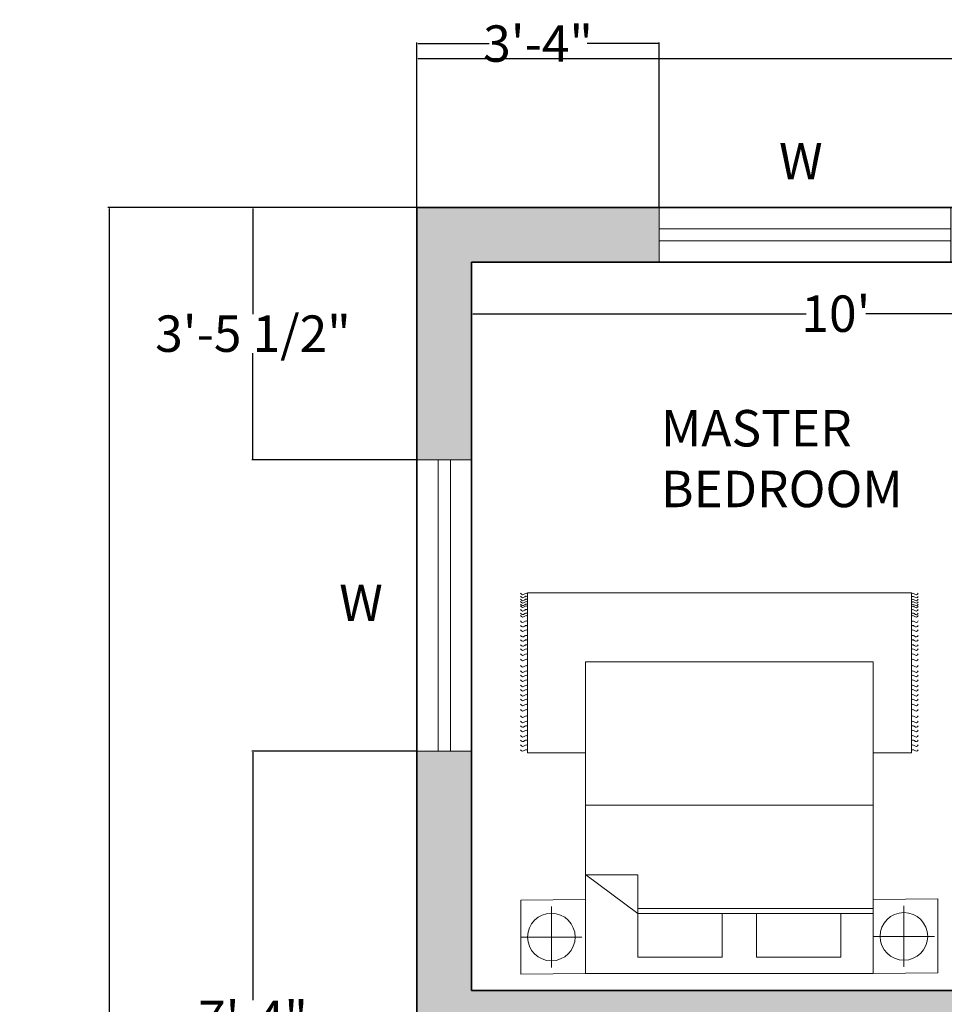
# Model space of a CAD drawing. Units: inches. Extents: x 302 to 1258, y 831 to 1373.
# Tile 3 of 13: x 302 to 455, y 1211 to 1373. Entities that reach past the tile are written whole.
import ezdxf

# ---------------------------------------------------------------- set-up
doc = ezdxf.new("R2010")
doc.units = ezdxf.units.IN
doc.header["$MEASUREMENT"] = 0
for name, color, linetype, lineweight in [('A-ANNO-DIMS', 2, 'Continuous', 18), ('A-ANNO-TEXT', 7, 'Continuous', 18), ('A-AREA-IDEN', 7, 'Continuous', 18), ('A-FURN', 8, 'Continuous', 18), ('A-GLAZ', 4, 'Continuous', 18), ('A-WALL', 7, 'Continuous', 35), ('A-WALL-PATT', 251, 'Continuous', 13)]:
    doc.layers.add(name, color=color, linetype=linetype, lineweight=lineweight)
doc.styles.get("Standard").update_dxf_attribs({"font": 'arial.ttf'})
doc.dimstyles.get("Standard").update_dxf_attribs({"dimtxt": 6, "dimasz": 0.18, "dimexe": 0.18, "dimexo": 0.0625, "dimgap": 0.09, "dimtad": 0, "dimtih": 1, "dimtoh": 1, "dimdec": 1, "dimzin": 0, "dimdsep": 46, "dimlunit": 3, "dimtxsty": 'Standard', "dimcen": 0.09, "dimadec": 0, "dimazin": 0, "dimtfac": 1, "dimtdec": 1, "dimtofl": 0, "dimtmove": 0, "dimatfit": 3, "dimfxl": 1, "dimtolj": 1, "dimtzin": 0, "dimarcsym": 0})

# ---------------------------------------------------------------- blocks, each defined once
blk = doc.blocks.new('*D3')
at = {"layer": 'A-ANNO-DIMS', "color": 0, "lineweight": -2, "transparency": 16777216}
for p, q in [((376.67, 1333.26), (376.67, 1324.65)), ((496.67, 1333.26), (496.67, 1324.65)), ((376.85, 1324.83), (431.77, 1324.83)), ((496.49, 1324.83), (441.57, 1324.83))]:
    blk.add_line(p, q, dxfattribs=at)
at = {"layer": 'A-ANNO-DIMS', "color": 0, "transparency": 16777216}
for points in [[(376.85, 1324.86), (376.85, 1324.8), (376.67, 1324.83)], [(496.49, 1324.86), (496.49, 1324.8), (496.67, 1324.83)]]:
    blk.add_solid(points, dxfattribs=at)
at = {"layer": 'Defpoints', "color": 0, "transparency": 16777216}
for p in [(376.67, 1333.32), (496.67, 1333.32), (496.67, 1324.83)]:
    blk.add_point(p, dxfattribs=at)
at = {"layer": 'A-ANNO-DIMS', "color": 0, "transparency": 16777216, "insert": (436.67, 1324.83), "char_height": 6, "attachment_point": 5}
blk.add_mtext("\\A1;10'", dxfattribs=at)
blk = doc.blocks.new('*D31')
at = {"layer": 'A-ANNO-DIMS', "color": 0, "lineweight": -2, "transparency": 16777216}
for p, q in [((367.67, 1342.38), (367.67, 1367.04)), ((367.85, 1366.86), (532.23, 1366.86)), ((724.49, 1366.86), (560.11, 1366.86)), ((724.67, 1342.38), (724.67, 1367.04))]:
    blk.add_line(p, q, dxfattribs=at)
at = {"layer": 'A-ANNO-DIMS', "color": 0, "transparency": 16777216}
for points in [[(367.85, 1366.89), (367.85, 1366.83), (367.67, 1366.86)], [(724.49, 1366.89), (724.49, 1366.83), (724.67, 1366.86)]]:
    blk.add_solid(points, dxfattribs=at)
at = {"layer": 'Defpoints', "color": 0, "transparency": 16777216}
for p in [(724.67, 1366.86), (367.67, 1342.32), (724.67, 1342.32)]:
    blk.add_point(p, dxfattribs=at)
at = {"layer": 'A-ANNO-DIMS', "color": 0, "transparency": 16777216, "insert": (546.17, 1366.86), "char_height": 6, "attachment_point": 5}
blk.add_mtext('\\A1;29\'-9.0"', dxfattribs=at)
blk = doc.blocks.new('*D32')
at = {"layer": 'A-ANNO-DIMS', "color": 0, "lineweight": -2, "transparency": 16777216}
for p, q in [((367.61, 1342.32), (316.79, 1342.32)), ((316.97, 1342.14), (316.97, 1107.72)), ((316.97, 867), (316.97, 1101.41)), ((367.61, 866.82), (316.79, 866.82))]:
    blk.add_line(p, q, dxfattribs=at)
at = {"layer": 'A-ANNO-DIMS', "color": 0, "transparency": 16777216}
for points in [[(316.94, 1342.14), (317, 1342.14), (316.97, 1342.32)], [(316.94, 867), (317, 867), (316.97, 866.82)]]:
    blk.add_solid(points, dxfattribs=at)
at = {"layer": 'Defpoints', "color": 0, "transparency": 16777216}
for p in [(367.67, 1342.32), (316.97, 866.82), (367.67, 866.82)]:
    blk.add_point(p, dxfattribs=at)
at = {"layer": 'A-ANNO-DIMS', "color": 0, "transparency": 16777216, "insert": (316.97, 1104.57), "char_height": 6, "attachment_point": 5}
blk.add_mtext('\\A1;39\'-7.5"', dxfattribs=at)
blk = doc.blocks.new('BED-DOUBLE-WITH-NIGHTSTANDS')
for p, q in [((1.12, 36.41), (1.12, 62.78)), ((1.12, 62.78), (64.36, 62.78)), ((64.36, 62.78), (64.36, 36.41)), ((10.66, 36.41), (1.12, 36.41)), ((64.36, 36.41), (58.06, 36.41)), ((10.66, 27.82), (58.08, 27.82)), ((19.27, 16.32), (10.71, 16.32)), ((19.32, 9.97), (10.71, 16.32)), ((19.27, 9.97), (19.27, 16.32)), ((5.06, 1.07), (5.06, 11.12)), ((19.27, 10.78), (58.08, 10.78)), ((19.32, 9.97), (58.08, 9.97)), ((63.11, 1.17), (63.11, 11.22)), ((0.03, 6.09), (10.09, 6.09)), ((58.08, 6.2), (68.14, 6.2))]:
    blk.add_line(p, q)
for points in [[(10.66, 0.1), (10.66, 51.42), (58.08, 51.42), (58.08, 0.1)], [(10.66, 12.29), (0.03, 12.19), (0.03, 0), (10.66, 0.1)], [(68.71, 12.39), (58.08, 12.29), (58.08, 0.1), (68.71, 0.2)], [(19.27, 2.8), (19.27, 9.97), (33.16, 9.97), (33.16, 2.8)], [(38.83, 2.8), (38.83, 9.97), (52.73, 9.97), (52.73, 2.8)]]:
    blk.add_lwpolyline(points, close=True)
for centre in [(5.06, 6.09), (63.11, 6.2)]:
    blk.add_circle(centre, 3.92)
for points, knots in [([(0, 62.71), (0.1, 62.59), (0.29, 62.35), (0.63, 62.59), (0.91, 62.76), (1.06, 62.66), (1.13, 62.61)], [0, 0, 0, 0, 0.400747, 0.791423, 1.067667, 1.29709, 1.29709, 1.29709, 1.29709]), ([(0, 62.24), (0.1, 62.12), (0.29, 61.88), (0.63, 62.12), (0.91, 62.29), (1.06, 62.18), (1.13, 62.13)], [0, 0, 0, 0, 0.400747, 0.791423, 1.067667, 1.29709, 1.29709, 1.29709, 1.29709]), ([(0, 61.75), (0.1, 61.63), (0.29, 61.39), (0.63, 61.63), (0.91, 61.8), (1.06, 61.7), (1.13, 61.65)], [0, 0, 0, 0, 0.400747, 0.791423, 1.067667, 1.29709, 1.29709, 1.29709, 1.29709]), ([(65.48, 62.71), (65.39, 62.59), (65.19, 62.35), (64.85, 62.59), (64.57, 62.76), (64.42, 62.66), (64.36, 62.61)], [0, 0, 0, 0, 0.400747, 0.791423, 1.067667, 1.29709, 1.29709, 1.29709, 1.29709]), ([(65.48, 62.21), (65.39, 62.09), (65.19, 61.85), (64.85, 62.09), (64.57, 62.26), (64.42, 62.15), (64.36, 62.11)], [0, 0, 0, 0, 0.400747, 0.791423, 1.067667, 1.29709, 1.29709, 1.29709, 1.29709]), ([(65.48, 61.72), (65.39, 61.6), (65.19, 61.36), (64.85, 61.6), (64.57, 61.78), (64.42, 61.67), (64.36, 61.62)], [0, 0, 0, 0, 0.400747, 0.791423, 1.067667, 1.29709, 1.29709, 1.29709, 1.29709]), ([(0, 61.35), (0.1, 61.23), (0.29, 60.99), (0.63, 61.23), (0.91, 61.41), (1.06, 61.3), (1.13, 61.25)], [0, 0, 0, 0, 0.400747, 0.791423, 1.067667, 1.29709, 1.29709, 1.29709, 1.29709]), ([(0, 60.94), (0.1, 60.81), (0.29, 60.58), (0.63, 60.81), (0.91, 60.99), (1.05, 60.89), (1.12, 60.84)], [0, 0, 0, 0, 0.400747, 0.791423, 1.067667, 1.283686, 1.283686, 1.283686, 1.283686]), ([(0, 60.63), (0.1, 60.51), (0.29, 60.27), (0.63, 60.51), (0.91, 60.68), (1.05, 60.58), (1.12, 60.53)], [0, 0, 0, 0, 0.400747, 0.791423, 1.067667, 1.283686, 1.283686, 1.283686, 1.283686]), ([(0, 60.05), (0.1, 59.93), (0.29, 59.69), (0.63, 59.93), (0.91, 60.1), (1.05, 60), (1.12, 59.96)], [0, 0, 0, 0, 0.400747, 0.791423, 1.067667, 1.283686, 1.283686, 1.283686, 1.283686]), ([(65.48, 61.33), (65.39, 61.21), (65.19, 60.97), (64.85, 61.21), (64.57, 61.38), (64.42, 61.27), (64.36, 61.22)], [0, 0, 0, 0, 0.400747, 0.791423, 1.067667, 1.29709, 1.29709, 1.29709, 1.29709]), ([(65.48, 60.91), (65.39, 60.79), (65.19, 60.55), (64.85, 60.79), (64.57, 60.96), (64.42, 60.85), (64.36, 60.81)], [0, 0, 0, 0, 0.400747, 0.791423, 1.067667, 1.29709, 1.29709, 1.29709, 1.29709]), ([(65.48, 60.6), (65.39, 60.48), (65.19, 60.24), (64.85, 60.48), (64.57, 60.65), (64.42, 60.54), (64.36, 60.5)], [0, 0, 0, 0, 0.400747, 0.791423, 1.067667, 1.29709, 1.29709, 1.29709, 1.29709]), ([(65.48, 60.03), (65.39, 59.9), (65.19, 59.67), (64.85, 59.9), (64.57, 60.08), (64.42, 59.97), (64.36, 59.92)], [0, 0, 0, 0, 0.400747, 0.791423, 1.067667, 1.29709, 1.29709, 1.29709, 1.29709]), ([(0, 59.46), (0.1, 59.34), (0.29, 59.09), (0.63, 59.34), (0.91, 59.51), (1.05, 59.41), (1.12, 59.36)], [0, 0, 0, 0, 0.402903, 0.794912, 1.071156, 1.287177, 1.287177, 1.287177, 1.287177]), ([(0, 59.03), (0.1, 58.91), (0.29, 58.67), (0.63, 58.91), (0.91, 59.08), (1.05, 58.98), (1.12, 58.93)], [0, 0, 0, 0, 0.400747, 0.791423, 1.067667, 1.283686, 1.283686, 1.283686, 1.283686]), ([(65.48, 59.46), (65.39, 59.33), (65.2, 59.08), (64.85, 59.34), (64.57, 59.51), (64.42, 59.4), (64.36, 59.36)], [0, 0, 0, 0, 0.407265, 0.802015, 1.07826, 1.307683, 1.307683, 1.307683, 1.307683]), ([(65.48, 59.03), (65.39, 58.91), (65.19, 58.67), (64.85, 58.91), (64.57, 59.08), (64.42, 58.97), (64.36, 58.93)], [0, 0, 0, 0, 0.400747, 0.791423, 1.067667, 1.29709, 1.29709, 1.29709, 1.29709]), ([(0, 58.15), (0.1, 58.03), (0.29, 57.79), (0.63, 58.03), (0.91, 58.2), (1.05, 58.1), (1.12, 58.05)], [0, 0, 0, 0, 0.400747, 0.791423, 1.067667, 1.283686, 1.283686, 1.283686, 1.283686]), ([(0, 57.42), (0.1, 57.3), (0.29, 57.06), (0.63, 57.3), (0.91, 57.47), (1.06, 57.36), (1.13, 57.32)], [0, 0, 0, 0, 0.400747, 0.791423, 1.067667, 1.29709, 1.29709, 1.29709, 1.29709]), ([(65.48, 58.15), (65.39, 58.03), (65.19, 57.79), (64.85, 58.03), (64.57, 58.2), (64.42, 58.09), (64.36, 58.04)], [0, 0, 0, 0, 0.400747, 0.791423, 1.067667, 1.29709, 1.29709, 1.29709, 1.29709]), ([(65.48, 57.42), (65.39, 57.3), (65.19, 57.06), (64.85, 57.3), (64.57, 57.47), (64.42, 57.36), (64.36, 57.32)], [0, 0, 0, 0, 0.400747, 0.791423, 1.067667, 1.29709, 1.29709, 1.29709, 1.29709]), ([(0, 56.67), (0.1, 56.55), (0.29, 56.31), (0.63, 56.55), (0.91, 56.72), (1.06, 56.61), (1.13, 56.56)], [0, 0, 0, 0, 0.400747, 0.791423, 1.067667, 1.29709, 1.29709, 1.29709, 1.29709]), ([(0, 55.78), (0.1, 55.66), (0.29, 55.42), (0.63, 55.66), (0.91, 55.84), (1.06, 55.73), (1.13, 55.68)], [0, 0, 0, 0, 0.400747, 0.791423, 1.067667, 1.29709, 1.29709, 1.29709, 1.29709]), ([(65.48, 56.67), (65.39, 56.55), (65.19, 56.31), (64.85, 56.55), (64.57, 56.72), (64.42, 56.61), (64.36, 56.56)], [0, 0, 0, 0, 0.400747, 0.791423, 1.067667, 1.29709, 1.29709, 1.29709, 1.29709]), ([(65.48, 55.78), (65.39, 55.66), (65.19, 55.42), (64.85, 55.66), (64.57, 55.84), (64.42, 55.73), (64.36, 55.68)], [0, 0, 0, 0, 0.400747, 0.791423, 1.067667, 1.29709, 1.29709, 1.29709, 1.29709]), ([(0, 55.06), (0.1, 54.94), (0.29, 54.7), (0.63, 54.94), (0.91, 55.11), (1.06, 55), (1.13, 54.95)], [0, 0, 0, 0, 0.400747, 0.791423, 1.067667, 1.29709, 1.29709, 1.29709, 1.29709]), ([(0, 54.24), (0.1, 54.12), (0.29, 53.88), (0.63, 54.12), (0.91, 54.29), (1.06, 54.19), (1.13, 54.14)], [0, 0, 0, 0, 0.400747, 0.791423, 1.067667, 1.29709, 1.29709, 1.29709, 1.29709]), ([(0, 53.55), (0.1, 53.43), (0.29, 53.19), (0.63, 53.43), (0.91, 53.6), (1.06, 53.5), (1.13, 53.45)], [0, 0, 0, 0, 0.400747, 0.791423, 1.067667, 1.29709, 1.29709, 1.29709, 1.29709]), ([(65.48, 55.06), (65.39, 54.94), (65.19, 54.7), (64.85, 54.94), (64.57, 55.11), (64.42, 55), (64.36, 54.95)], [0, 0, 0, 0, 0.400747, 0.791423, 1.067667, 1.29709, 1.29709, 1.29709, 1.29709]), ([(65.48, 54.24), (65.39, 54.12), (65.19, 53.88), (64.85, 54.12), (64.57, 54.29), (64.42, 54.19), (64.36, 54.14)], [0, 0, 0, 0, 0.400747, 0.791423, 1.067667, 1.29709, 1.29709, 1.29709, 1.29709]), ([(65.48, 53.55), (65.39, 53.43), (65.19, 53.19), (64.85, 53.43), (64.57, 53.6), (64.42, 53.5), (64.36, 53.45)], [0, 0, 0, 0, 0.400747, 0.791423, 1.067667, 1.29709, 1.29709, 1.29709, 1.29709]), ([(0, 52.73), (0.1, 52.61), (0.29, 52.37), (0.63, 52.61), (0.91, 52.79), (1.06, 52.68), (1.13, 52.63)], [0, 0, 0, 0, 0.400747, 0.791423, 1.067667, 1.29709, 1.29709, 1.29709, 1.29709]), ([(65.48, 52.73), (65.39, 52.61), (65.19, 52.37), (64.85, 52.61), (64.57, 52.79), (64.42, 52.68), (64.36, 52.63)], [0, 0, 0, 0, 0.400747, 0.791423, 1.067667, 1.29709, 1.29709, 1.29709, 1.29709]), ([(0, 51.85), (0.1, 51.73), (0.29, 51.49), (0.63, 51.73), (0.91, 51.9), (1.06, 51.8), (1.13, 51.75)], [0, 0, 0, 0, 0.400747, 0.791423, 1.067667, 1.29709, 1.29709, 1.29709, 1.29709]), ([(0, 50.82), (0.1, 50.69), (0.29, 50.46), (0.63, 50.69), (0.91, 50.87), (1.06, 50.76), (1.13, 50.71)], [0, 0, 0, 0, 0.400747, 0.791423, 1.067667, 1.29709, 1.29709, 1.29709, 1.29709]), ([(65.48, 51.85), (65.39, 51.73), (65.19, 51.49), (64.85, 51.73), (64.57, 51.9), (64.42, 51.8), (64.36, 51.75)], [0, 0, 0, 0, 0.400747, 0.791423, 1.067667, 1.29709, 1.29709, 1.29709, 1.29709]), ([(65.48, 50.82), (65.39, 50.69), (65.19, 50.46), (64.85, 50.69), (64.57, 50.87), (64.42, 50.76), (64.36, 50.71)], [0, 0, 0, 0, 0.400747, 0.791423, 1.067667, 1.29709, 1.29709, 1.29709, 1.29709]), ([(0, 49.93), (0.1, 49.81), (0.29, 49.57), (0.63, 49.81), (0.91, 49.99), (1.06, 49.88), (1.13, 49.83)], [0, 0, 0, 0, 0.400747, 0.791423, 1.067667, 1.29709, 1.29709, 1.29709, 1.29709]), ([(0, 49.21), (0.1, 49.08), (0.29, 48.84), (0.63, 49.08), (0.91, 49.26), (1.06, 49.15), (1.13, 49.1)], [0, 0, 0, 0, 0.400747, 0.791423, 1.067667, 1.29709, 1.29709, 1.29709, 1.29709]), ([(65.48, 49.93), (65.39, 49.81), (65.19, 49.57), (64.85, 49.81), (64.57, 49.99), (64.42, 49.88), (64.36, 49.83)], [0, 0, 0, 0, 0.400747, 0.791423, 1.067667, 1.29709, 1.29709, 1.29709, 1.29709]), ([(65.48, 49.21), (65.39, 49.08), (65.19, 48.84), (64.85, 49.08), (64.57, 49.26), (64.42, 49.15), (64.36, 49.1)], [0, 0, 0, 0, 0.400747, 0.791423, 1.067667, 1.29709, 1.29709, 1.29709, 1.29709]), ([(0, 48.45), (0.1, 48.33), (0.29, 48.09), (0.63, 48.33), (0.91, 48.51), (1.06, 48.4), (1.13, 48.35)], [0, 0, 0, 0, 0.400747, 0.791423, 1.067667, 1.29709, 1.29709, 1.29709, 1.29709]), ([(0, 47.57), (0.1, 47.45), (0.29, 47.21), (0.63, 47.45), (0.91, 47.62), (1.06, 47.52), (1.13, 47.47)], [0, 0, 0, 0, 0.400747, 0.791423, 1.067667, 1.29709, 1.29709, 1.29709, 1.29709]), ([(65.48, 48.45), (65.39, 48.33), (65.19, 48.09), (64.85, 48.33), (64.57, 48.51), (64.42, 48.4), (64.36, 48.35)], [0, 0, 0, 0, 0.400747, 0.791423, 1.067667, 1.29709, 1.29709, 1.29709, 1.29709]), ([(65.48, 47.57), (65.39, 47.45), (65.19, 47.21), (64.85, 47.45), (64.57, 47.62), (64.42, 47.52), (64.36, 47.47)], [0, 0, 0, 0, 0.400747, 0.791423, 1.067667, 1.29709, 1.29709, 1.29709, 1.29709]), ([(0, 46.84), (0.1, 46.72), (0.29, 46.48), (0.63, 46.72), (0.91, 46.89), (1.06, 46.79), (1.13, 46.74)], [0, 0, 0, 0, 0.400747, 0.791423, 1.067667, 1.29709, 1.29709, 1.29709, 1.29709]), ([(0, 46.03), (0.1, 45.91), (0.29, 45.67), (0.63, 45.91), (0.91, 46.08), (1.06, 45.97), (1.13, 45.92)], [0, 0, 0, 0, 0.400747, 0.791423, 1.067667, 1.29709, 1.29709, 1.29709, 1.29709]), ([(65.48, 46.84), (65.39, 46.72), (65.19, 46.48), (64.85, 46.72), (64.57, 46.89), (64.42, 46.79), (64.36, 46.74)], [0, 0, 0, 0, 0.400747, 0.791423, 1.067667, 1.29709, 1.29709, 1.29709, 1.29709]), ([(65.48, 46.03), (65.39, 45.91), (65.19, 45.67), (64.85, 45.91), (64.57, 46.08), (64.42, 45.97), (64.36, 45.92)], [0, 0, 0, 0, 0.400747, 0.791423, 1.067667, 1.29709, 1.29709, 1.29709, 1.29709]), ([(0, 45.25), (0.1, 45.13), (0.29, 44.89), (0.63, 45.13), (0.91, 45.3), (1.06, 45.2), (1.13, 45.15)], [0, 0, 0, 0, 0.400747, 0.791423, 1.067667, 1.29709, 1.29709, 1.29709, 1.29709]), ([(0, 44.43), (0.1, 44.31), (0.29, 44.07), (0.63, 44.31), (0.91, 44.49), (1.06, 44.38), (1.13, 44.33)], [0, 0, 0, 0, 0.400747, 0.791423, 1.067667, 1.29709, 1.29709, 1.29709, 1.29709]), ([(65.48, 45.25), (65.39, 45.13), (65.19, 44.89), (64.85, 45.13), (64.57, 45.3), (64.42, 45.2), (64.36, 45.15)], [0, 0, 0, 0, 0.400747, 0.791423, 1.067667, 1.29709, 1.29709, 1.29709, 1.29709]), ([(65.48, 44.43), (65.39, 44.31), (65.19, 44.07), (64.85, 44.31), (64.57, 44.49), (64.42, 44.38), (64.36, 44.33)], [0, 0, 0, 0, 0.400747, 0.791423, 1.067667, 1.29709, 1.29709, 1.29709, 1.29709]), ([(0, 43.55), (0.1, 43.43), (0.29, 43.19), (0.63, 43.43), (0.91, 43.6), (1.06, 43.5), (1.13, 43.45)], [0, 0, 0, 0, 0.400747, 0.791423, 1.067667, 1.29709, 1.29709, 1.29709, 1.29709]), ([(0, 42.52), (0.1, 42.39), (0.29, 42.15), (0.63, 42.39), (0.91, 42.57), (1.06, 42.46), (1.13, 42.41)], [0, 0, 0, 0, 0.400747, 0.791423, 1.067667, 1.29709, 1.29709, 1.29709, 1.29709]), ([(65.48, 43.55), (65.39, 43.43), (65.19, 43.19), (64.85, 43.43), (64.57, 43.6), (64.42, 43.5), (64.36, 43.45)], [0, 0, 0, 0, 0.400747, 0.791423, 1.067667, 1.29709, 1.29709, 1.29709, 1.29709]), ([(65.48, 42.52), (65.39, 42.39), (65.19, 42.15), (64.85, 42.39), (64.57, 42.57), (64.42, 42.46), (64.36, 42.41)], [0, 0, 0, 0, 0.400747, 0.791423, 1.067667, 1.29709, 1.29709, 1.29709, 1.29709]), ([(0, 41.63), (0.1, 41.51), (0.29, 41.27), (0.63, 41.51), (0.91, 41.68), (1.06, 41.58), (1.13, 41.53)], [0, 0, 0, 0, 0.400747, 0.791423, 1.067667, 1.29709, 1.29709, 1.29709, 1.29709]), ([(0, 40.9), (0.1, 40.78), (0.29, 40.54), (0.63, 40.78), (0.91, 40.96), (1.06, 40.85), (1.13, 40.8)], [0, 0, 0, 0, 0.400747, 0.791423, 1.067667, 1.29709, 1.29709, 1.29709, 1.29709]), ([(65.48, 41.63), (65.39, 41.51), (65.19, 41.27), (64.85, 41.51), (64.57, 41.68), (64.42, 41.58), (64.36, 41.53)], [0, 0, 0, 0, 0.400747, 0.791423, 1.067667, 1.29709, 1.29709, 1.29709, 1.29709]), ([(65.48, 40.9), (65.39, 40.78), (65.19, 40.54), (64.85, 40.78), (64.57, 40.96), (64.42, 40.85), (64.36, 40.8)], [0, 0, 0, 0, 0.400747, 0.791423, 1.067667, 1.29709, 1.29709, 1.29709, 1.29709]), ([(0, 40.15), (0.1, 40.03), (0.29, 39.79), (0.63, 40.03), (0.91, 40.2), (1.06, 40.1), (1.13, 40.05)], [0, 0, 0, 0, 0.400747, 0.791423, 1.067667, 1.29709, 1.29709, 1.29709, 1.29709]), ([(0, 39.27), (0.1, 39.15), (0.29, 38.91), (0.63, 39.15), (0.91, 39.32), (1.06, 39.22), (1.13, 39.17)], [0, 0, 0, 0, 0.400747, 0.791423, 1.067667, 1.29709, 1.29709, 1.29709, 1.29709]), ([(65.48, 40.15), (65.39, 40.03), (65.19, 39.79), (64.85, 40.03), (64.57, 40.2), (64.42, 40.1), (64.36, 40.05)], [0, 0, 0, 0, 0.400747, 0.791423, 1.067667, 1.29709, 1.29709, 1.29709, 1.29709]), ([(65.48, 39.27), (65.39, 39.15), (65.19, 38.91), (64.85, 39.15), (64.57, 39.32), (64.42, 39.22), (64.36, 39.17)], [0, 0, 0, 0, 0.400747, 0.791423, 1.067667, 1.29709, 1.29709, 1.29709, 1.29709]), ([(0, 38.54), (0.1, 38.42), (0.29, 38.18), (0.63, 38.42), (0.91, 38.59), (1.06, 38.49), (1.13, 38.44)], [0, 0, 0, 0, 0.400747, 0.791423, 1.067667, 1.29709, 1.29709, 1.29709, 1.29709]), ([(0, 37.73), (0.1, 37.61), (0.29, 37.37), (0.63, 37.61), (0.91, 37.78), (1.06, 37.67), (1.13, 37.62)], [0, 0, 0, 0, 0.400747, 0.791423, 1.067667, 1.29709, 1.29709, 1.29709, 1.29709]), ([(65.48, 38.54), (65.39, 38.42), (65.19, 38.18), (64.85, 38.42), (64.57, 38.59), (64.42, 38.49), (64.36, 38.44)], [0, 0, 0, 0, 0.400747, 0.791423, 1.067667, 1.29709, 1.29709, 1.29709, 1.29709]), ([(65.48, 37.73), (65.39, 37.61), (65.19, 37.37), (64.85, 37.61), (64.57, 37.78), (64.42, 37.67), (64.36, 37.62)], [0, 0, 0, 0, 0.400747, 0.791423, 1.067667, 1.29709, 1.29709, 1.29709, 1.29709]), ([(0, 36.95), (0.1, 36.83), (0.29, 36.59), (0.63, 36.83), (0.91, 37), (1.06, 36.89), (1.13, 36.85)], [0, 0, 0, 0, 0.400747, 0.791423, 1.067667, 1.29709, 1.29709, 1.29709, 1.29709]), ([(65.48, 36.95), (65.39, 36.83), (65.19, 36.59), (64.85, 36.83), (64.57, 37), (64.42, 36.89), (64.36, 36.85)], [0, 0, 0, 0, 0.400747, 0.791423, 1.067667, 1.29709, 1.29709, 1.29709, 1.29709])]:
    blk.add_open_spline(points, degree=3, knots=knots)
blk = doc.blocks.new('WINDOW-48IN')
for p, q in [((0, 0), (0, 9)), ((0, 9), (48, 9)), ((48, 9), (48, 0)), ((0, 5.5), (48, 5.5)), ((48, 3.5), (0, 3.5)), ((48, 0), (0, 0))]:
    blk.add_line(p, q)
blk = doc.blocks.new('*D69')
at = {"layer": 'A-ANNO-DIMS', "color": 0, "lineweight": -2, "transparency": 16777216}
for p, q in [((367.67, 1342.38), (367.67, 1369.5)), ((367.85, 1369.32), (379.56, 1369.32)), ((407.39, 1369.32), (395.68, 1369.32)), ((407.57, 1342.38), (407.57, 1369.5))]:
    blk.add_line(p, q, dxfattribs=at)
at = {"layer": 'A-ANNO-DIMS', "color": 0, "transparency": 16777216}
for points in [[(367.85, 1369.35), (367.85, 1369.29), (367.67, 1369.32)], [(407.39, 1369.35), (407.39, 1369.29), (407.57, 1369.32)]]:
    blk.add_solid(points, dxfattribs=at)
at = {"layer": 'Defpoints', "color": 0, "transparency": 16777216}
for p in [(407.57, 1369.32), (367.67, 1342.32), (407.57, 1342.32)]:
    blk.add_point(p, dxfattribs=at)
at = {"layer": 'A-ANNO-DIMS', "color": 0, "transparency": 16777216, "insert": (387.62, 1369.32), "char_height": 6, "attachment_point": 5}
blk.add_mtext('\\A1;3\'-4"', dxfattribs=at)
blk = doc.blocks.new('*D71')
at = {"layer": 'A-ANNO-DIMS', "color": 0, "lineweight": -2, "transparency": 16777216}
for p, q in [((367.61, 1342.32), (340.49, 1342.32)), ((340.67, 1342.14), (340.67, 1324.73)), ((340.67, 1300.94), (340.67, 1318.34)), ((367.61, 1300.76), (340.49, 1300.76))]:
    blk.add_line(p, q, dxfattribs=at)
at = {"layer": 'A-ANNO-DIMS', "color": 0, "transparency": 16777216}
for points in [[(340.64, 1342.14), (340.7, 1342.14), (340.67, 1342.32)], [(340.64, 1300.94), (340.7, 1300.94), (340.67, 1300.76)]]:
    blk.add_solid(points, dxfattribs=at)
at = {"layer": 'Defpoints', "color": 0, "transparency": 16777216}
for p in [(367.67, 1342.32), (340.67, 1300.76), (367.67, 1300.76)]:
    blk.add_point(p, dxfattribs=at)
at = {"layer": 'A-ANNO-DIMS', "color": 0, "transparency": 16777216, "insert": (340.67, 1321.54), "char_height": 6, "attachment_point": 5}
blk.add_mtext('\\A1;3\'-5 1/2"', dxfattribs=at)
blk = doc.blocks.new('*D72')
at = {"layer": 'A-ANNO-DIMS', "color": 0, "lineweight": -2, "transparency": 16777216}
for p, q in [((367.60766, 1252.758966), (340.49016, 1252.758966)), ((340.67016, 1252.578966), (340.67016, 1211.744211)), ((340.67016, 1164.729456), (340.67016, 1205.564211)), ((367.60766, 1164.549456), (340.49016, 1164.549456))]:
    blk.add_line(p, q, dxfattribs=at)
at = {"layer": 'A-ANNO-DIMS', "color": 0, "transparency": 16777216}
for points in [[(340.64016, 1252.578966), (340.70016, 1252.578966), (340.67016, 1252.758966)], [(340.64016, 1164.729456), (340.70016, 1164.729456), (340.67016, 1164.549456)]]:
    blk.add_solid(points, dxfattribs=at)
at = {"layer": 'Defpoints', "color": 0, "transparency": 16777216}
for p in [(367.67016, 1252.758966), (340.67016, 1164.549456), (367.67016, 1164.549456)]:
    blk.add_point(p, dxfattribs=at)
at = {"layer": 'A-ANNO-DIMS', "color": 0, "transparency": 16777216, "insert": (340.67016, 1208.654211), "char_height": 6, "attachment_point": 5}
blk.add_mtext('\\A1;7\'-4"', dxfattribs=at)

msp = doc.modelspace()

# ---------------------------------------------------------------- hatches: boundary and pattern name
at = {"layer": 'A-WALL-PATT'}
h = msp.add_hatch(color=256, dxfattribs=at)
h.dxf.hatch_style = 1
h.paths.add_polyline_path([(524.78, 1342.32), (455.57, 1342.32), (455.57, 1333.32), (496.67, 1333.32), (496.67, 1330.32), (501.17, 1330.32), (501.17, 1333.32), (524.78, 1333.32)])
h.paths.add_polyline_path([(724.67, 1342.32), (548.78, 1342.32), (548.78, 1333.32), (567.17, 1333.32), (567.17, 1213.32), (501.17, 1213.32), (501.17, 1306.32), (496.67, 1306.32), (496.67, 1213.32), (495.67, 1213.32), (495.67, 1208.82), (496.67, 1208.82), (572.67, 1208.82), (572.67, 1213.32), (571.67, 1213.32), (571.67, 1333.32), (715.67, 1333.32), (715.67, 1302.71), (724.67, 1302.71)])
h.paths.add_polyline_path([(376.67, 1333.32), (407.57, 1333.32), (407.57, 1342.32), (367.67, 1342.32), (367.67, 1300.76), (376.67, 1300.76)])
h.paths.add_polyline_path([(459.67, 1213.32), (376.67, 1213.32), (376.67, 1252.76), (367.67, 1252.76), (367.67, 1164.55), (376.67, 1164.55), (376.67, 1208.82), (454.67, 1208.82), (454.67, 1082.82), (459.17, 1082.82), (459.17, 1208.82), (459.67, 1208.82)])
h.paths.add_polyline_path([(376.67, 1116.55), (367.67, 1116.55), (367.67, 1024.44), (376.67, 1024.44)])
h.paths.add_polyline_path([(724.67, 1254.71), (715.67, 1254.71), (715.67, 1213.32), (608.67, 1213.32), (608.67, 1208.82), (615.17, 1208.82), (615.17, 1205.82), (619.67, 1205.82), (619.67, 1208.82), (715.67, 1208.82), (715.67, 1191.3), (724.67, 1191.3)])
h.paths.add_polyline_path([(724.67, 1167.3), (715.67, 1167.3), (715.67, 1136.82), (619.67, 1136.82), (619.67, 1181.82), (615.17, 1181.82), (615.17, 1136.82), (591.17, 1136.82), (591.17, 1129.32), (595.67, 1129.32), (595.67, 1132.32), (715.67, 1132.32), (715.67, 1097.42), (724.67, 1097.42)])
h.paths.add_polyline_path([(724.67, 1049.42), (715.67, 1049.42), (715.67, 1012.32), (595.67, 1012.32), (595.67, 1093.32), (591.17, 1093.32), (591.17, 1007.82), (715.67, 1007.82), (715.67, 875.82), (709.67, 875.82), (709.67, 866.82), (715.67, 866.82), (724.67, 866.82)])
h.paths.add_polyline_path([(673.67, 875.82), (623.88, 875.82), (623.88, 866.82), (673.67, 866.82)], flags=17)
h.paths.add_polyline_path([(575.88, 875.82), (477.17, 875.82), (477.17, 971.82), (472.67, 971.82), (472.67, 875.82), (376.67, 875.82), (376.67, 896.2), (367.67, 896.2), (367.67, 866.82), (575.88, 866.82)])
h.paths.add_polyline_path([(376.67, 976.44), (367.67, 976.44), (367.67, 944.2), (376.67, 944.2)])

# ---------------------------------------------------------------- linework, layer by layer
at = {"layer": 'A-WALL'}
for p, q in [((367.67, 1342.32), (724.67, 1342.32)), ((367.67, 1342.32), (367.67, 866.82)), ((376.67, 1333.32), (376.67, 1213.32)), ((376.67, 1333.32), (496.67, 1333.32)), ((376.67, 1213.32), (459.67, 1213.32))]:
    msp.add_line(p, q, dxfattribs=at)

# ---------------------------------------------------------------- block references
at = {"layer": 'A-FURN'}
msp.add_blockref('BED-DOUBLE-WITH-NIGHTSTANDS', (384.75, 1216.06), dxfattribs=at)
at = {"layer": 'A-GLAZ'}
msp.add_blockref('WINDOW-48IN', (407.57, 1333.32), dxfattribs=at)
at = {"layer": 'A-GLAZ', "rotation": 269.9999999999997}
msp.add_blockref('WINDOW-48IN', (367.67, 1300.76), dxfattribs=at)

# ---------------------------------------------------------------- texts
at = {"layer": 'A-ANNO-TEXT', "char_height": 6, "attachment_point": 1}
for insert in [(427.3, 1352.94), (354.87, 1280.2)]:
    msp.add_mtext_dynamic_manual_height_columns('W', width=16.4894, gutter_width=30, heights=[0], dxfattribs=dict(at, insert=insert))
at = {"layer": 'A-AREA-IDEN', "insert": (407.85, 1308.96), "char_height": 6, "attachment_point": 1}
msp.add_mtext_dynamic_manual_height_columns('MASTER\\PBEDROOM', width=60.4741, gutter_width=30, heights=[0], dxfattribs=at)

# ---------------------------------------------------------------- dimensions: what is measured, and where the dimension line sits
at = {"layer": 'A-ANNO-DIMS'}
for base, p1, p2, override, picture, middle in [((407.57, 1369.32), (367.67, 1342.32), (407.57, 1342.32), {"dimdec": 1, "dimlfac": 1, "dimrnd": 0, "dimzin": 1, "dimdsep": 46, "dimlunit": 4, "dimfrac": 2}, '*D69', (387.62, 1369.32)), ((724.67, 1366.86), (367.67, 1342.32), (724.67, 1342.32), {"dimclrd": 0, "dimclre": 0, "dimclrt": 0}, '*D31', (546.17, 1366.86)), ((496.67, 1324.83), (376.67, 1333.32), (496.67, 1333.32), {"dimclrd": 0, "dimclre": 0, "dimclrt": 0}, '*D3', (436.67, 1324.83))]:
    dim = msp.add_linear_dim(base=base, p1=p1, p2=p2, dimstyle='Standard', override=override, dxfattribs=at)
    dim.commit()
    dim.dimension.update_dxf_attribs({"geometry": picture, "text_midpoint": middle})
for base, p1, p2, override, picture, middle in [((316.97, 866.82), (367.67, 1342.32), (367.67, 866.82), {"dimclrd": 0, "dimclre": 0, "dimclrt": 0}, '*D32', (316.97, 1104.57)), ((340.67, 1300.76), (367.67, 1342.32), (367.67, 1300.76), {"dimdec": 1, "dimlfac": 1, "dimrnd": 0, "dimzin": 1, "dimdsep": 46, "dimlunit": 4, "dimfrac": 2}, '*D71', (340.67, 1321.54)), ((340.67, 1164.55), (367.67, 1252.76), (367.67, 1164.55), {"dimdec": 1, "dimlfac": 1, "dimrnd": 0, "dimzin": 1, "dimdsep": 46, "dimlunit": 4, "dimfrac": 2}, '*D72', (340.67, 1208.65))]:
    dim = msp.add_linear_dim(base=base, p1=p1, p2=p2, angle=90, dimstyle='Standard', override=override, dxfattribs=at)
    dim.commit()
    dim.dimension.update_dxf_attribs({"geometry": picture, "text_midpoint": middle})

doc.saveas('drawing.dxf')
